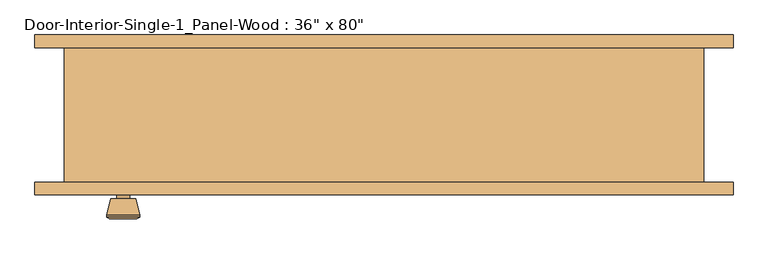
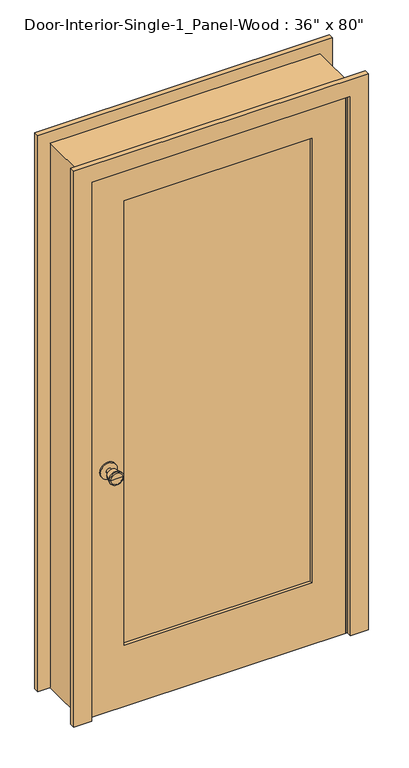
"""IFC4 building model written with IfcOpenShell, lengths in millimetres: door geometry."""

from ifc_helpers import new_model, si_unit, point, frame, frame_2d, origin, place, context, project, spatial, polyline, circle_curve, trimmed, segment, composite_curve, outline, extrude, faceted_brep, source, transform, mapped, element, save
from ifc_brep_helpers import plane_surface, cylinder_surface, revolved_surface, advanced_brep


def door_89b565b6(model_context):
    return source(origin(), model_context, "Body", "SolidModel", [
        advanced_brep(
        [(-393.7, -57.5, 914.4), (-403.7, -57.5, 914.4), (-383.7, -57.5, 914.4), (-373.2241324, -8.5, 914.4), (-414.1758676, -8.5, 914.4), (-393.7, -8.5, 914.4), (-368.7, -10.3278681, 914.4), (-418.7, -10.3278681, 914.4), (-368.7, -13.7915463, 914.4), (-418.7, -13.7915463, 914.4), (-375.063764, -38.5, 914.4), (-412.336236, -38.5, 914.4), (-383.7, -38.5, 914.4), (-403.7, -38.5, 914.4)],
        [
            (0, 1),
            (1, 2, circle_curve(frame((-393.7, -57.5, 914.4), z_axis=(0.0, -1.0, 0.0), x_axis=(-1.0, 0.0, 0.0)), 10.0)),
            (2, 0),
            (2, 1, circle_curve(frame((-393.7, -57.5, 914.4), z_axis=(0.0, -1.0, 0.0), x_axis=(-1.0, 0.0, 0.0)), 10.0)),
            (3, 4, circle_curve(frame((-393.7, -8.5, 914.4), z_axis=(0.0, 1.0, 0.0), x_axis=(-1.0, 0.0, 0.0)), 20.4758676)),
            (4, 5),
            (5, 3),
            (4, 3, circle_curve(frame((-393.7, -8.5, 914.4), z_axis=(0.0, 1.0, 0.0), x_axis=(-1.0, 0.0, 0.0)), 20.4758676)),
            (6, 7, circle_curve(frame((-393.7, -10.3278681, 914.4), z_axis=(0.0, 1.0, 0.0), x_axis=(-1.0, 0.0, 0.0)), 25.0)),
            (7, 4),
            (3, 6),
            (7, 6, circle_curve(frame((-393.7, -10.3278681, 914.4), z_axis=(0.0, 1.0, 0.0), x_axis=(-1.0, 0.0, 0.0)), 25.0)),
            (8, 9, circle_curve(frame((-393.7, -13.7915463, 914.4), z_axis=(0.0, 1.0, 0.0), x_axis=(-1.0, 0.0, 0.0)), 25.0)),
            (9, 7),
            (6, 8),
            (9, 8, circle_curve(frame((-393.7, -13.7915463, 914.4), z_axis=(0.0, 1.0, 0.0), x_axis=(-1.0, 0.0, 0.0)), 25.0)),
            (10, 11, circle_curve(frame((-393.7, -38.5, 914.4), z_axis=(0.0, 1.0, 0.0), x_axis=(-1.0, 0.0, 0.0)), 18.636236)),
            (11, 9),
            (8, 10),
            (11, 10, circle_curve(frame((-393.7, -38.5, 914.4), z_axis=(0.0, 1.0, 0.0), x_axis=(-1.0, 0.0, 0.0)), 18.636236)),
            (12, 13, circle_curve(frame((-393.7, -38.5, 914.4), z_axis=(0.0, 1.0, 0.0), x_axis=(-1.0, 0.0, 0.0)), 10.0)),
            (13, 11),
            (10, 12),
            (13, 12, circle_curve(frame((-393.7, -38.5, 914.4), z_axis=(0.0, 1.0, 0.0), x_axis=(-1.0, 0.0, 0.0)), 10.0)),
            (1, 13),
            (12, 2),
        ],
        [
            plane_surface(frame((-393.7, -57.5, 914.4), z_axis=(0.0, -1.0, 0.0), x_axis=(-1.0, 0.0, 0.0))),
            plane_surface(frame((-393.7, -8.5, 914.4), z_axis=(0.0, 1.0, 0.0), x_axis=(-1.0, 0.0, 0.0))),
            revolved_surface(polyline([(-414.1758676, -8.5, 914.4), (-418.7, -10.3278681, 914.4)]), (-393.7, -57.5, 914.4), (0.0, -1.0, 0.0)),
            cylinder_surface(frame((-393.7, -57.5, 914.4), z_axis=(0.0, -1.0, 0.0), x_axis=(-1.0, 0.0, 0.0)), 25.0),
            revolved_surface(polyline([(-418.7, -13.7915463, 914.4), (-412.336236, -38.5, 914.4)]), (-393.7, -57.5, 914.4), (0.0, -1.0, 0.0)),
            plane_surface(frame((-393.7, -38.5, 914.4), z_axis=(0.0, -1.0, 0.0), x_axis=(-1.0, 0.0, 0.0))),
            cylinder_surface(frame((-393.7, -57.5, 914.4), z_axis=(0.0, -1.0, 0.0), x_axis=(-1.0, 0.0, 0.0)), 10.0),
        ],
        [
            (0, [[1, 2, 3]]),
            (0, [[-3, 4, -1]]),
            (1, [[5, 6, 7]]),
            (1, [[8, -7, -6]]),
            (2, [[9, 10, -5, 11]]),
            (2, [[12, -11, -8, -10]]),
            (3, [[13, 14, -9, 15]]),
            (3, [[16, -15, -12, -14]]),
            (4, [[17, 18, -13, 19]]),
            (4, [[20, -19, -16, -18]]),
            (5, [[21, 22, -17, 23]]),
            (5, [[24, -23, -20, -22]]),
            (6, [[-2, 25, -21, 26]]),
            (6, [[-4, -26, -24, -25]]),
        ],
    ),
        extrude(outline(composite_curve([segment(trimmed(circle_curve(frame_2d((914.4, -393.7)), 30.0), [point((914.4, -423.7))], [point((914.4, -363.7))], False, "CARTESIAN"), True, "CONTINUOUS"), segment(trimmed(circle_curve(frame_2d((914.4, -393.7)), 30.0), [point((914.4, -363.7))], [point((914.4, -423.7))], False, "CARTESIAN"), True, "CONTINUOUS")], self_intersect=False)), frame((0.0, -63.5, 0.0), z_axis=(0.0, 1.0, 0.0), x_axis=(0.0, 0.0, 1.0)), (0.0, 0.0, 1.0), 6.0),
        advanced_brep(
        [(-393.7, -104.425, 914.4), (-383.7, -104.425, 914.4), (-403.7, -104.425, 914.4), (-373.2241324, -153.425, 914.4), (-393.7, -153.425, 914.4), (-414.1758676, -153.425, 914.4), (-368.7, -151.5971319, 914.4), (-418.7, -151.5971319, 914.4), (-368.7, -148.1334537, 914.4), (-418.7, -148.1334537, 914.4), (-375.063764, -123.425, 914.4), (-412.336236, -123.425, 914.4), (-383.7, -123.425, 914.4), (-403.7, -123.425, 914.4)],
        [
            (0, 1),
            (1, 2, circle_curve(frame((-393.7, -104.425, 914.4), z_axis=(0.0, 1.0, 0.0), x_axis=(-1.0, 0.0, 0.0)), 10.0)),
            (2, 0),
            (2, 1, circle_curve(frame((-393.7, -104.425, 914.4), z_axis=(0.0, 1.0, 0.0), x_axis=(-1.0, 0.0, 0.0)), 10.0)),
            (3, 4),
            (4, 5),
            (5, 3, circle_curve(frame((-393.7, -153.425, 914.4), z_axis=(0.0, -1.0, 0.0), x_axis=(-1.0, 0.0, 0.0)), 20.4758676)),
            (3, 5, circle_curve(frame((-393.7, -153.425, 914.4), z_axis=(0.0, -1.0, 0.0), x_axis=(-1.0, 0.0, 0.0)), 20.4758676)),
            (6, 3),
            (5, 7),
            (7, 6, circle_curve(frame((-393.7, -151.5971319, 914.4), z_axis=(0.0, -1.0, 0.0), x_axis=(-1.0, 0.0, 0.0)), 25.0)),
            (6, 7, circle_curve(frame((-393.7, -151.5971319, 914.4), z_axis=(0.0, -1.0, 0.0), x_axis=(-1.0, 0.0, 0.0)), 25.0)),
            (8, 6),
            (7, 9),
            (9, 8, circle_curve(frame((-393.7, -148.1334537, 914.4), z_axis=(0.0, -1.0, 0.0), x_axis=(-1.0, 0.0, 0.0)), 25.0)),
            (8, 9, circle_curve(frame((-393.7, -148.1334537, 914.4), z_axis=(0.0, -1.0, 0.0), x_axis=(-1.0, 0.0, 0.0)), 25.0)),
            (10, 8),
            (9, 11),
            (11, 10, circle_curve(frame((-393.7, -123.425, 914.4), z_axis=(0.0, -1.0, 0.0), x_axis=(-1.0, 0.0, 0.0)), 18.636236)),
            (10, 11, circle_curve(frame((-393.7, -123.425, 914.4), z_axis=(0.0, -1.0, 0.0), x_axis=(-1.0, 0.0, 0.0)), 18.636236)),
            (12, 10),
            (11, 13),
            (13, 12, circle_curve(frame((-393.7, -123.425, 914.4), z_axis=(0.0, -1.0, 0.0), x_axis=(-1.0, 0.0, 0.0)), 10.0)),
            (12, 13, circle_curve(frame((-393.7, -123.425, 914.4), z_axis=(0.0, -1.0, 0.0), x_axis=(-1.0, 0.0, 0.0)), 10.0)),
            (1, 12),
            (13, 2),
        ],
        [
            plane_surface(frame((-393.7, -104.425, 914.4), z_axis=(0.0, 1.0, 0.0), x_axis=(-1.0, 0.0, 0.0))),
            plane_surface(frame((-393.7, -153.425, 914.4), z_axis=(0.0, -1.0, 0.0), x_axis=(-1.0, 0.0, 0.0))),
            revolved_surface(polyline([(-414.1758676, -153.425, 914.4), (-418.7, -151.5971319, 914.4)]), (-393.7, -104.425, 914.4), (0.0, 1.0, 0.0)),
            cylinder_surface(frame((-393.7, -104.425, 914.4), z_axis=(0.0, 1.0, 0.0), x_axis=(-1.0, 0.0, 0.0)), 25.0),
            revolved_surface(polyline([(-418.7, -148.1334537, 914.4), (-412.336236, -123.425, 914.4)]), (-393.7, -104.425, 914.4), (0.0, 1.0, 0.0)),
            plane_surface(frame((-393.7, -123.425, 914.4), z_axis=(0.0, 1.0, 0.0), x_axis=(-1.0, 0.0, 0.0))),
            cylinder_surface(frame((-393.7, -104.425, 914.4), z_axis=(0.0, 1.0, 0.0), x_axis=(-1.0, 0.0, 0.0)), 10.0),
        ],
        [
            (0, [[1, 2, 3]]),
            (0, [[-3, 4, -1]]),
            (1, [[5, 6, 7]]),
            (1, [[-6, -5, 8]]),
            (2, [[9, -7, 10, 11]]),
            (2, [[-10, -8, -9, 12]]),
            (3, [[13, -11, 14, 15]]),
            (3, [[-14, -12, -13, 16]]),
            (4, [[17, -15, 18, 19]]),
            (4, [[-18, -16, -17, 20]]),
            (5, [[21, -19, 22, 23]]),
            (5, [[-22, -20, -21, 24]]),
            (6, [[25, -23, 26, -2]]),
            (6, [[-26, -24, -25, -4]]),
        ],
    ),
        extrude(outline(composite_curve([segment(trimmed(circle_curve(frame_2d((914.4, -393.7)), 30.0), [point((914.4, -423.7))], [point((914.4, -363.7))], False, "CARTESIAN"), True, "CONTINUOUS"), segment(trimmed(circle_curve(frame_2d((914.4, -393.7)), 30.0), [point((914.4, -363.7))], [point((914.4, -423.7))], False, "CARTESIAN"), True, "CONTINUOUS")], self_intersect=False)), frame((0.0, -104.425, 0.0), z_axis=(0.0, 1.0, 0.0), x_axis=(0.0, 0.0, 1.0)), (0.0, 0.0, 1.0), 6.0),
        faceted_brep([(482.6, -98.425, 0.0), (457.2, -98.425, 0.0), (457.2, -63.5, 0.0), (444.5, -63.5, 0.0), (444.5, -28.575, 0.0), (457.2, -28.575, 0.0), (457.2, 104.775, 0.0), (482.6, 104.775, 0.0), (482.6, 104.775, 2057.4), (482.6, -98.425, 2057.4), (457.2, 104.775, 2032.0), (-457.2, 104.775, 2032.0), (-457.2, 104.775, 0.0), (-482.6, 104.775, 0.0), (-482.6, 104.775, 2057.4), (457.2, -28.575, 2032.0), (444.5, -28.575, 2019.3), (-444.5, -28.575, 2019.3), (-444.5, -28.575, 0.0), (-457.2, -28.575, 0.0), (-457.2, -28.575, 2032.0), (444.5, -63.5, 2019.3), (457.2, -63.5, 2032.0), (-457.2, -63.5, 2032.0), (-457.2, -63.5, 0.0), (-444.5, -63.5, 0.0), (-444.5, -63.5, 2019.3), (457.2, -98.425, 2032.0), (-482.6, -98.425, 2057.4), (-482.6, -98.425, 0.0), (-457.2, -98.425, 0.0), (-457.2, -98.425, 2032.0)], [[[0, 1, 2, 3, 4, 5, 6, 7]], [[7, 8, 9, 0]], [[6, 10, 11, 12, 13, 14, 8, 7]], [[5, 15, 10, 6]], [[4, 16, 17, 18, 19, 20, 15, 5]], [[3, 21, 16, 4]], [[2, 22, 23, 24, 25, 26, 21, 3]], [[1, 27, 22, 2]], [[0, 9, 28, 29, 30, 31, 27, 1]], [[8, 14, 28, 9]], [[15, 20, 11, 10]], [[21, 26, 17, 16]], [[27, 31, 23, 22]], [[29, 13, 12, 19, 18, 25, 24, 30]], [[14, 13, 29, 28]], [[20, 19, 12, 11]], [[26, 25, 18, 17]], [[31, 30, 24, 23]]]),
        extrude(outline(polyline([(2032.0, -457.2), (0.0, -457.2), (0.0, 457.2), (2032.0, 457.2), (2032.0, -457.2)]), holes=[polyline([(1912.9375, -336.55), (1912.9375, 336.55), (231.775, 336.55), (231.775, -336.55), (1912.9375, -336.55)])]), frame((0.0, -98.425, 0.0), z_axis=(0.0, 1.0, 0.0), x_axis=(0.0, 0.0, 1.0)), (0.0, 0.0, 1.0), 34.925),
        extrude(outline(polyline([(336.55, -75.1416667), (336.55, -86.7833333), (-336.55, -86.7833333), (-336.55, -75.1416667), (336.55, -75.1416667)])), frame((0.0, 0.0, 231.775), z_axis=(0.0, 0.0, 1.0), x_axis=(1.0, 0.0, 0.0)), (0.0, 0.0, 1.0), 1681.1625),
        extrude(outline(polyline([(0.0, 527.05), (2101.85, 527.05), (2101.85, -527.05), (0.0, -527.05), (0.0, -463.55), (2038.35, -463.55), (2038.35, 463.55), (0.0, 463.55), (0.0, 527.05)])), frame((0.0, -117.475, 0.0), z_axis=(0.0, 1.0, 0.0), x_axis=(0.0, 0.0, 1.0)), (0.0, 0.0, 1.0), 19.05),
        extrude(outline(polyline([(0.0, 527.05), (2101.85, 527.05), (2101.85, -527.05), (0.0, -527.05), (0.0, -463.55), (2038.35, -463.55), (2038.35, 463.55), (0.0, 463.55), (0.0, 527.05)])), frame((0.0, 104.775, 0.0), z_axis=(0.0, 1.0, 0.0), x_axis=(0.0, 0.0, 1.0)), (0.0, 0.0, 1.0), 19.05),
    ])


if __name__ == "__main__":
    model = new_model("IFC4")
    model_context = context("Model", 3, world=origin())
    ifc_project = project(units=[si_unit("LENGTHUNIT", "METRE", prefix="MILLI")], contexts=[model_context])
    site = spatial("IfcSite", under=ifc_project)
    building = spatial("IfcBuilding", under=site)
    placement = place(None, origin())
    door_shape = door_89b565b6(model_context)
    element("IfcDoor", 1, ObjectType="Door-Interior-Single-1_Panel-Wood : 36\" x 80\"", at=placement, inside=building, context=model_context, shape_type="MappedRepresentation", body=[
        mapped(door_shape, transform((0.0, 0.0, 0.0), x_axis=(1.0, 0.0, 0.0), y_axis=(0.0, 1.0, 0.0), z_axis=(0.0, 0.0, 1.0))),
    ])
    save(model, "model.ifc")

# Revit data of these elements
# Type "Door-Interior-Single-1_Panel-Wood : 36\" x 80\""
#   Type Mark = "10"
#   Assembly Code = "C1020300"
#   Analytic Construction = "Wooden"
#   Top Rail = 0' - 4 11/16"
#   Thickness = 0' - 1 3/8"
#   Thermal Resistance (R) = 2.5876 (h·ft²·°F)/BTU
#   Swing Angle [instance default] = 90.00°
#   Stiles = 0' - 4 3/4"
#   Rough Width = 3' - 2"
#   Rough Height = 6' - 9"
#   Height = 6' - 8"
#   Width = 3' - 0"
#   Heat Transfer Coefficient (U) = 0.3865 BTU/(h·ft²·°F)
#   Bottom Rail = 0' - 9 1/8"
#   Trim Material = Cherry
#   Panel Material = Cherry
#   Frame Material = Cherry
#   Door Handle Material = Aluminum
#   Visual Light Transmittance = 0
#   Solar Heat Gain Coefficient = 0
#   Wall Closure = (empty or 0)
#   Function = (empty or 0)
# Element 1 (IfcDoor, "Door-Interior-Single-1_Panel-Wood : 36\" x 80\"")
#   Materials on its faces: "Cherry", "Aluminum"
# Materials
#   "Cherry": class "Wood", colour RGB 226 177 128, transparency 0, Description = "Prunus Serotina", Cost = 0
#   "Aluminum": class "Metal", colour RGB 247 247 247, transparency 0, Description = "Aluminum 6061", Cost = 0
